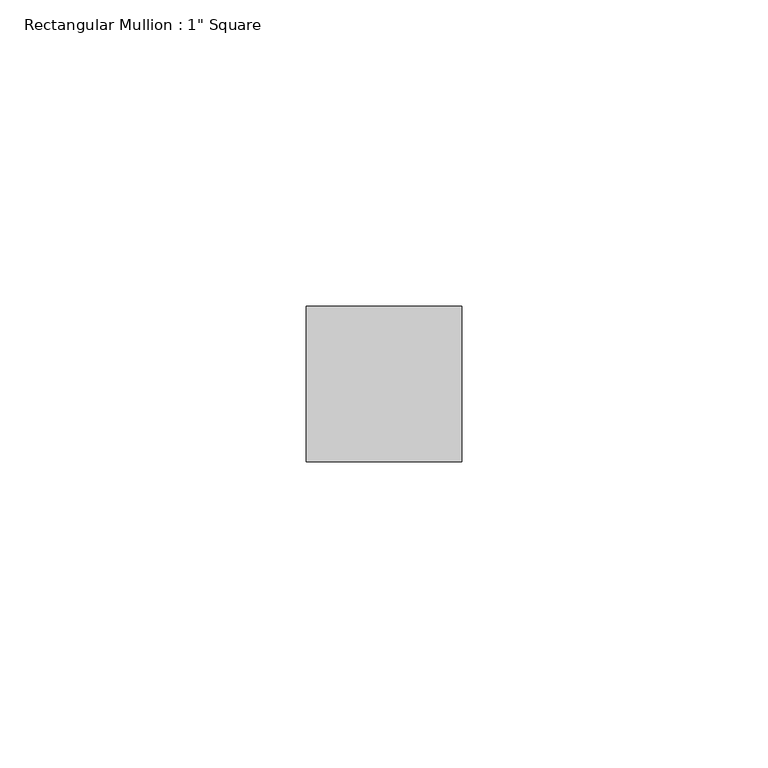
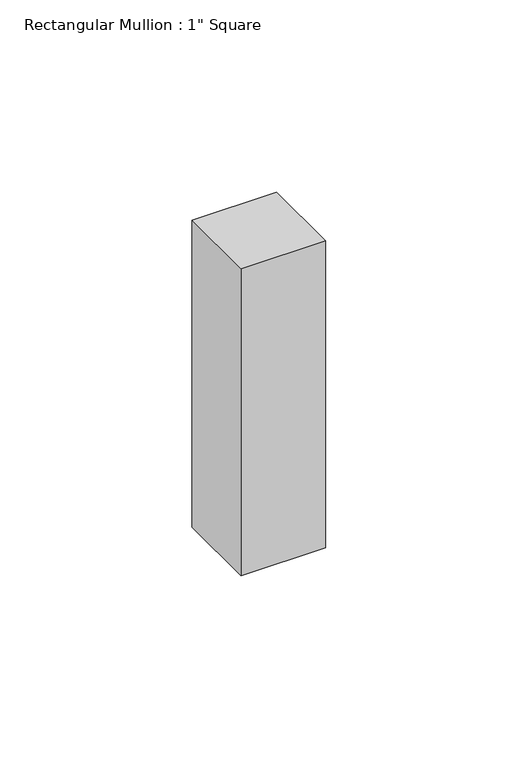
"""IFC4 building model written with IfcOpenShell, lengths in millimetres: member geometry."""

from ifc_helpers import new_model, si_unit, frame, origin, place, context, project, spatial, polyline, outline, extrude, source, transform, mapped, element, save


def member_dc9417da(model_context):
    return source(origin(), model_context, "Body", "SweptSolid", [
        extrude(outline(polyline([(0.0, 12.7), (0.0, -12.7), (-25.4, -12.7), (-25.4, 12.7), (0.0, 12.7)])), frame((0.0, 0.0, -97.3666667), z_axis=(0.0, 0.0, 1.0), x_axis=(1.0, 0.0, 0.0)), (0.0, 0.0, 1.0), 97.3666667),
    ])


if __name__ == "__main__":
    model = new_model("IFC4")
    model_context = context("Model", 3, world=origin())
    ifc_project = project(units=[si_unit("LENGTHUNIT", "METRE", prefix="MILLI")], contexts=[model_context])
    site = spatial("IfcSite", under=ifc_project)
    building = spatial("IfcBuilding", under=site)
    placement = place(None, origin())
    member_shape = member_dc9417da(model_context)
    element("IfcMember", 1, ObjectType="Rectangular Mullion : 1\" Square", at=placement, inside=building, context=model_context, shape_type="MappedRepresentation", body=[
        mapped(member_shape, transform((0.0, 0.0, 0.0), x_axis=(1.0, 0.0, 0.0), y_axis=(0.0, 1.0, 0.0), z_axis=(0.0, 0.0, 1.0))),
    ])
    save(model, "model.ifc")

# Revit data of these elements
# Type "Rectangular Mullion : 1\" Square"
#   built-in parameter 1007304 = 0.0833333 (stored number, unit not read)
#   built-in parameter 1007301 = 0.0416667 (stored number, unit not read)
#   built-in parameter 1007300 = 0.0416667 (stored number, unit not read)
# Element 1 (IfcMember, "Rectangular Mullion : 1\" Square")
#   Materials on its faces: "black"
# Materials
#   "black": class "Generic", colour RGB 120 120 120, transparency 0, Cost = 0
